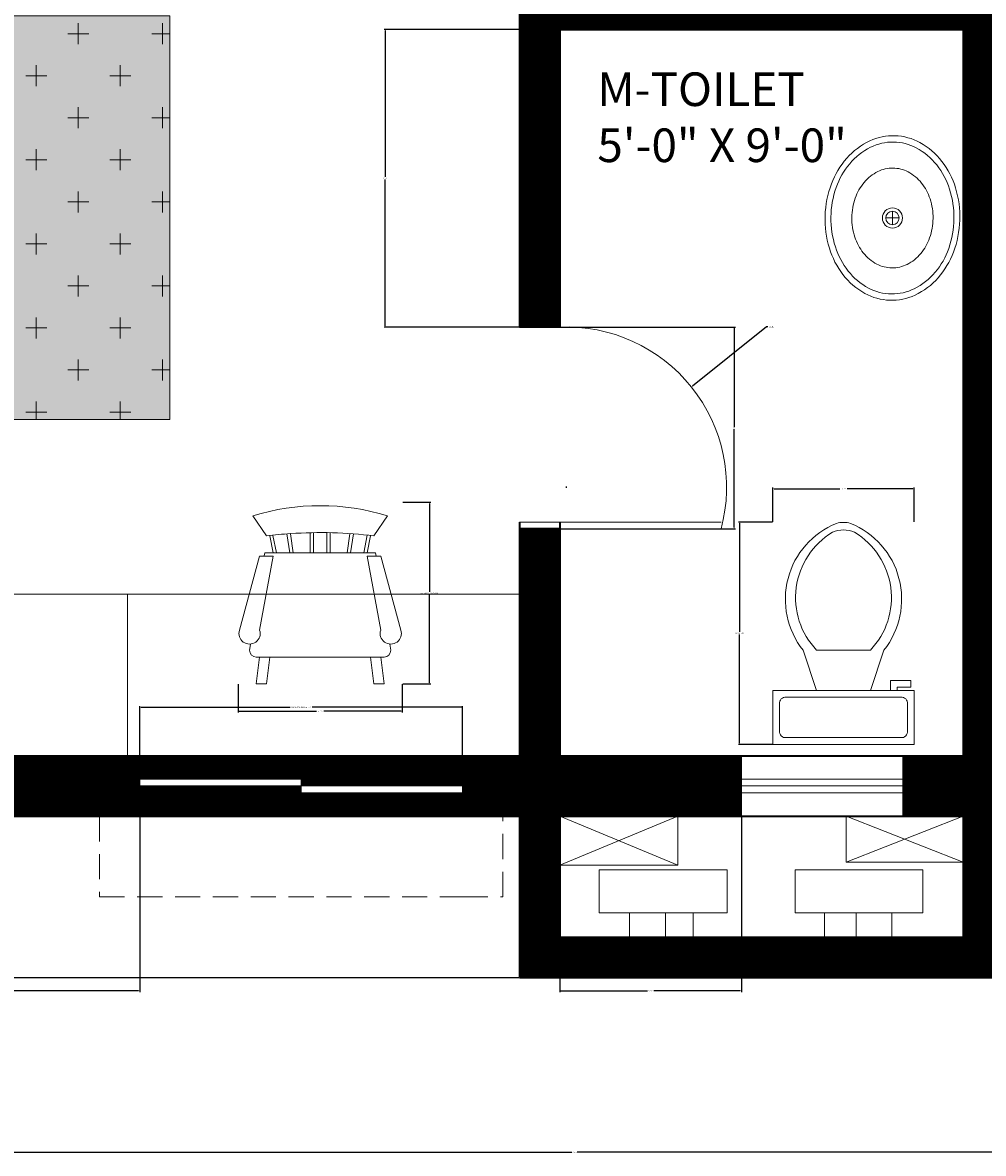
# Model space of a CAD drawing. Units: inches. Extents: x 557 to 1007, y 390 to 953.
# Tile 2 of 10: x 700 to 842, y 390 to 558. Entities that reach past the tile are written whole.
import ezdxf

# ---------------------------------------------------------------- set-up
doc = ezdxf.new("R2010")
doc.units = ezdxf.units.IN
doc.header["$LTSCALE"] = 5
doc.header["$MEASUREMENT"] = 0
doc.linetypes.add('HIDDEN', pattern=[0.375, 0.25, -0.125])
for name, color, linetype, lineweight in [('A-ANNO-DIMS', 2, 'Continuous', 18), ('A-AREA-IDEN', 7, 'Continuous', 18), ('A-DOOR', 3, 'Continuous', 18), ('A-EQPM', 8, 'Continuous', 18), ('A-FLOR-CASE', 8, 'Continuous', 18), ('A-FLOR-FIXT', 9, 'Continuous', 18), ('A-FURN', 8, 'Continuous', 18), ('A-FURN-PATT', 9, 'Continuous', 9), ('A-GLAZ', 4, 'Continuous', 18), ('A-GLAZ-OVHD', 8, 'HIDDEN', 13), ('A-WALL', 7, 'Continuous', 35)]:
    doc.layers.add(name, color=color, linetype=linetype, lineweight=lineweight)
doc.layers.add('A-GLAZ-PATT', color=141, linetype='Continuous', lineweight=9, true_color=0xadddf7)
doc.layers.add('A-WALL-PATT', color=251, linetype='Continuous', lineweight=9, true_color=0x636466)
doc.styles.get("Standard").update_dxf_attribs({"font": 'arial.ttf'})
doc.dimstyles.get("Standard").update_dxf_attribs({"dimtxt": 0.18, "dimasz": 0.18, "dimexe": 0.18, "dimexo": 0.0625, "dimgap": 0.09, "dimtad": 0, "dimtih": 1, "dimtoh": 1, "dimdec": 4, "dimzin": 0, "dimdsep": 46, "dimtxsty": 'Standard', "dimcen": 0.09, "dimadec": 0, "dimazin": 0, "dimtfac": 1, "dimtdec": 4, "dimtofl": 0, "dimtmove": 0, "dimatfit": 3, "dimfxl": 1, "dimtolj": 1, "dimtzin": 0, "dimarcsym": 0})

# ---------------------------------------------------------------- blocks, each defined once
blk = doc.blocks.new('Chair - Rocking')
for p, q in [((-8, -4.5), (-10, -1.5)), ((8, -4.5), (10, -1.5)), ((-7.5, -4.5), (-7, -7)), ((-6.5, -7), (-7.02225, -4.43)), ((-4.5, -7), (-4.96674, -4.19951)), ((-4, -7), (-4.40532, -4.16272)), ((-1.5, -4.05012), (-1.5, -7)), ((-1, -7), (-1, -4.05012)), ((1, -7), (1, -4.04655)), ((1.5, -4.05012), (1.5, -7)), ((4, -7), (4.40187, -4.18694)), ((4.5, -7), (4.96761, -4.19437)), ((6.5, -7), (7, -4.4057)), ((7.5, -4.5), (7, -7)), ((-9, -7.5), (-12, -18.49999)), ((-7, -7.5), (-9, -7.5)), ((-9, -18.49999), (-7, -7.5)), ((-8.23428, -6.99939), (-8.3093, -7.47958)), ((-8.23041, -7), (8.23915, -7)), ((7, -7.5), (9, -7.5)), ((9, -18.49999), (7, -7.5)), ((8.31071, -7.48854), (8.23449, -7.00073)), ((9, -7.5), (12, -18.49999)), ((-10.36644, -20.64523), (-10.5, -21.49999)), ((10.5, -21.49999), (10.3575, -20.58798)), ((-9, -22.49999), (-9.5, -26.49999)), ((0, -22.49999), (-9.5, -22.49999)), ((-8, -26.49999), (-7.5, -22.49999)), ((0, -22.49999), (9.5, -22.49999)), ((8, -26.49999), (7.5, -22.49999)), ((9, -22.49999), (9.5, -26.49999)), ((-9.5, -26.49999), (-8, -26.49999)), ((9.5, -26.49999), (8, -26.49999))]:
    blk.add_line(p, q)
for centre, radius, start, end in [((0, -34.08333), 34.08333, 72.93847, 107.0615), ((0, -68.25004), 64.25, 93.92211, 97.15267), ((0, -68.25004), 64.25, 82.84733, 93.92211), ((-10.5, -18.99999), 1.58114, 161.5651, 18.43495), ((10.5, -18.99999), 1.58114, 161.5651, 18.43495), ((-9.5, -21.49999), 1, 180, 270), ((9.5, -21.49999), 1, 270, 0)]:
    blk.add_arc(centre, radius, start, end)
blk = doc.blocks.new('Toilet - top')
for p, q in [((9.5, -6), (9.5, -2)), ((-8, -8.5), (-8, -8)), ((-7, -8), (-7, -9.5)), ((-4, -8), (-6, -14)), ((4, -8), (6, -14)), ((-10, -8.5), (-8, -8.5)), ((-10, -9.5), (-10, -8.5)), ((-7, -9.5), (-10, -9.5)), ((4, -14), (-4, -14))]:
    blk.add_line(p, q)
blk.add_lwpolyline([(10.5, -8), (10.5, 0), (-10.5, 0), (-10.5, -8)], close=True)
for points in [[(8.5, -1), (-8.5, -1)], [(-9.5, -2), (-9.5, -6)], [(-8.5, -7), (8.5, -7)]]:
    blk.add_lwpolyline(points)
for centre, radius, start, end in [((-8.62, -1.88), 0.884, 81.8699, 188.1301), ((8.62, -1.88), 0.884, 351.8699, 98.1301), ((-8.62, -6.12), 0.884, 171.8699, 278.1301), ((8.62, -6.12), 0.884, 261.8699, 8.1301), ((3.52, -21.58), 12.17, 141.4691, 247.9714), ((4.2, -21.82), 11.33, 136.3677, 238.9468), ((-3.52, -21.58), 12.17, 292.0284, 38.5307), ((-4.2, -21.82), 11.33, 301.053, 43.6321), ((0, -27.88), 4, 245.7318, 294.2682), ((0, -29), 4, 254.8605, 285.1395)]:
    blk.add_arc(centre, radius, start, end)
blk = doc.blocks.new('Sink - Oval top')
for p, q in [((-1, 0), (1, 0)), ((0, 1), (0, -1))]:
    blk.add_line(p, q)
for points in [[(-12.23, 0.39, 0.117634), (-11.46, -3.36, 0.104469), (-8.88, -6.8, 0.090016), (-5.08, -9.07, 0.08192), (-0.32, -10.02, 0.08192), (4.49, -9.38, 0.090016), (8.42, -7.36, 0.104469), (11.22, -4.09, 0.117634), (12.23, -0.39, 0.117634), (11.46, 3.36, 0.104469), (8.88, 6.8, 0.090016), (5.08, 9.07, 0.08192), (0.32, 10.02, 0.08192), (-4.49, 9.38, 0.090016), (-8.42, 7.36, 0.104469), (-11.22, 4.09, 0.117634)], [(-11.29, 0.16, 0.118622), (-10.52, -3.25, 0.104678), (-8.07, -6.36, 0.089562), (-4.54, -8.37, 0.081185), (-0.13, -9.15, 0.081185), (4.3, -8.49, 0.089562), (7.89, -6.58, 0.104678), (10.42, -3.55, 0.118622), (11.29, -0.16, 0.118622), (10.52, 3.25, 0.104678), (8.07, 6.36, 0.089562), (4.54, 8.37, 0.081185), (0.13, 9.15, 0.081185), (-4.3, 8.49, 0.089562), (-7.89, 6.58, 0.104678), (-10.42, 3.55, 0.118622)], [(-7.42, 0.08, 0.118283), (-6.91, -2.17, 0.104607), (-5.29, -4.21, 0.089718), (-2.97, -5.53, 0.081436), (-0.07, -6.04, 0.081436), (2.84, -5.59, 0.089718), (5.2, -4.33, 0.104607), (6.86, -2.32, 0.118283), (7.42, -0.08, 0.118283), (6.91, 2.17, 0.104607), (5.29, 4.21, 0.089718), (2.97, 5.53, 0.081436), (0.07, 6.04, 0.081436), (-2.84, 5.59, 0.089718), (-5.2, 4.33, 0.104607), (-6.86, 2.32, 0.118283)]]:
    blk.add_lwpolyline(points, format="xyb", close=True)
for radius in [1.5, 1]:
    blk.add_circle((0, 0), radius)
blk = doc.blocks.new('BED-QUEEN-60x80-PLAN')
for p, q in [((0, 0), (0, 60)), ((0, 60), (80, 60)), ((29.6, 60), (14.4, 44.8)), ((29.6, 44.8), (29.6, 60)), ((80, 60), (80, 0)), ((1.2, 52), (16.4, 52)), ((1.2, 31.2), (1.2, 52)), ((16.4, 52), (16.4, 46.8)), ((14.4, 0), (14.4, 44.8)), ((14.4, 44.8), (29.6, 44.8)), ((16.8, 44.8), (16.8, 0)), ((14.4, 31.2), (1.2, 31.2)), ((1.2, 28.8), (14.4, 28.8)), ((1.2, 8), (1.2, 28.8)), ((14.4, 8), (1.2, 8)), ((80, 0), (0, 0))]:
    blk.add_line(p, q)
blk = doc.blocks.new('WIN-24-VENT')
for p, q in [((0, 0), (0, 9)), ((24, 0), (24, 9)), ((24, 5.5), (0, 5.5)), ((24, 4.5), (0, 4.5)), ((24, 3.5), (0, 3.5))]:
    blk.add_line(p, q)
blk = doc.blocks.new('WIN-48-SLIDING')
for p, q in [((0, 9), (0, 0)), ((48, 9), (48, 0)), ((24, 5.5), (0, 5.5)), ((24, 5.5), (24, 3.5)), ((48, 4.5), (0, 4.5)), ((48, 3.5), (24, 3.5))]:
    blk.add_line(p, q)
blk = doc.blocks.new('WINDOW-SHADE-60')
at = {"ltscale": 3}
for p, q in [((12, 60), (0, 60)), ((0, 60), (0, 6)), ((12, 54), (12, 60)), ((0, 6), (0, 0)), ((0, 0), (12, 0))]:
    blk.add_line(p, q, dxfattribs=at)
blk = doc.blocks.new('*D23')
at = {"layer": 'A-ANNO-DIMS', "color": 0, "lineweight": -2, "ltscale": 5, "transparency": 16777216}
for p, q in [((756.06, 486.58), (760.23, 486.58)), ((760.05, 486.4), (760.05, 473.26)), ((760.05, 459.76), (760.05, 472.9)), ((756.06, 459.58), (760.23, 459.58))]:
    blk.add_line(p, q, dxfattribs=at)
at = {"layer": 'A-ANNO-DIMS', "color": 0, "ltscale": 5, "transparency": 16777216}
for points in [[(760.02, 486.4), (760.08, 486.4), (760.05, 486.58)], [(760.02, 459.76), (760.08, 459.76), (760.05, 459.58)]]:
    blk.add_solid(points, dxfattribs=at)
at = {"layer": 'Defpoints', "color": 0, "ltscale": 5, "transparency": 16777216}
for p in [(756, 486.58), (760.05, 486.58), (756, 459.58)]:
    blk.add_point(p, dxfattribs=at)
at = {"layer": 'A-ANNO-DIMS', "color": 0, "ltscale": 5, "transparency": 16777216, "insert": (760.05, 473.08), "char_height": 0.18, "attachment_point": 5}
blk.add_mtext('\\A1;ROCKING CHAIR 27 TYP.', dxfattribs=at)
blk = doc.blocks.new('*D24')
at = {"layer": 'A-ANNO-DIMS', "color": 0, "lineweight": -2, "ltscale": 5, "transparency": 16777216}
for p, q in [((731.57, 459.52), (731.57, 455.35)), ((756, 459.52), (756, 455.35)), ((731.75, 455.53), (743.26, 455.53)), ((755.82, 455.53), (744.31, 455.53))]:
    blk.add_line(p, q, dxfattribs=at)
at = {"layer": 'A-ANNO-DIMS', "color": 0, "ltscale": 5, "transparency": 16777216}
for points in [[(731.75, 455.56), (731.75, 455.5), (731.57, 455.53)], [(755.82, 455.56), (755.82, 455.5), (756, 455.53)]]:
    blk.add_solid(points, dxfattribs=at)
at = {"layer": 'Defpoints', "color": 0, "ltscale": 5, "transparency": 16777216}
for p in [(731.57, 459.58), (756, 459.58), (756, 455.53)]:
    blk.add_point(p, dxfattribs=at)
at = {"layer": 'A-ANNO-DIMS', "color": 0, "ltscale": 5, "transparency": 16777216, "insert": (743.78, 455.53), "char_height": 0.18, "attachment_point": 5}
blk.add_mtext('\\A1;24 TYP.', dxfattribs=at)
blk = doc.blocks.new('*D29')
at = {"layer": 'A-ANNO-DIMS', "color": 0, "lineweight": -2, "ltscale": 5, "transparency": 16777216}
for p, q in [((811.04, 483.64), (805.97, 483.64)), ((806.15, 483.46), (806.15, 467.3)), ((806.15, 450.77), (806.15, 466.93)), ((811.04, 450.59), (805.97, 450.59))]:
    blk.add_line(p, q, dxfattribs=at)
at = {"layer": 'A-ANNO-DIMS', "color": 0, "ltscale": 5, "transparency": 16777216}
for points in [[(806.12, 483.46), (806.18, 483.46), (806.15, 483.64)], [(806.12, 450.77), (806.18, 450.77), (806.15, 450.59)]]:
    blk.add_solid(points, dxfattribs=at)
at = {"layer": 'Defpoints', "color": 0, "ltscale": 5, "transparency": 16777216}
for p in [(811.1, 483.64), (806.15, 450.59), (811.1, 450.59)]:
    blk.add_point(p, dxfattribs=at)
at = {"layer": 'A-ANNO-DIMS', "color": 0, "ltscale": 5, "transparency": 16777216, "insert": (806.15, 467.11), "char_height": 0.18, "attachment_point": 5}
blk.add_mtext('\\A1;WC 33 TYP.', dxfattribs=at)
blk = doc.blocks.new('*D30')
at = {"layer": 'A-ANNO-DIMS', "color": 0, "lineweight": -2, "ltscale": 5, "transparency": 16777216}
for p, q in [((811.1, 483.7), (811.1, 488.77)), ((811.28, 488.59), (821.07, 488.59)), ((831.92, 488.59), (822.13, 488.59)), ((832.1, 483.7), (832.1, 488.77))]:
    blk.add_line(p, q, dxfattribs=at)
at = {"layer": 'A-ANNO-DIMS', "color": 0, "ltscale": 5, "transparency": 16777216}
for points in [[(811.28, 488.62), (811.28, 488.56), (811.1, 488.59)], [(831.92, 488.62), (831.92, 488.56), (832.1, 488.59)]]:
    blk.add_solid(points, dxfattribs=at)
at = {"layer": 'Defpoints', "color": 0, "ltscale": 5, "transparency": 16777216}
for p in [(811.1, 488.59), (811.1, 483.64), (832.1, 483.64)]:
    blk.add_point(p, dxfattribs=at)
at = {"layer": 'A-ANNO-DIMS', "color": 0, "ltscale": 5, "transparency": 16777216, "insert": (821.6, 488.59), "char_height": 0.18, "attachment_point": 5}
blk.add_mtext('\\A1;21 TYP.', dxfattribs=at)
blk = doc.blocks.new('*D33')
at = {"layer": 'A-ANNO-DIMS', "color": 0, "lineweight": -2, "ltscale": 5, "transparency": 16777216}
for p, q in [((716.96, 448.97), (716.96, 456.28)), ((717.14, 456.1), (739.31, 456.1)), ((764.78, 456.1), (742.61, 456.1)), ((764.96, 448.97), (764.96, 456.28))]:
    blk.add_line(p, q, dxfattribs=at)
at = {"layer": 'A-ANNO-DIMS', "color": 0, "ltscale": 5, "transparency": 16777216}
for points in [[(717.14, 456.13), (717.14, 456.07), (716.96, 456.1)], [(764.78, 456.13), (764.78, 456.07), (764.96, 456.1)]]:
    blk.add_solid(points, dxfattribs=at)
at = {"layer": 'Defpoints', "color": 0, "ltscale": 5, "transparency": 16777216}
for p in [(764.96, 456.1), (716.96, 448.9), (764.96, 448.9)]:
    blk.add_point(p, dxfattribs=at)
at = {"layer": 'A-ANNO-DIMS', "color": 0, "ltscale": 5, "transparency": 16777216, "insert": (740.96, 456.1), "char_height": 0.18, "attachment_point": 5}
blk.add_mtext('\\A1;SLIDING WINDOW 48 TYP.', dxfattribs=at)
blk = doc.blocks.new('*D34')
at = {"layer": 'A-ANNO-DIMS', "color": 0, "lineweight": -2, "ltscale": 5, "transparency": 16777216}
for p, q in [((716.9, 448.9), (709.58, 448.9)), ((709.76, 448.72), (709.76, 444.59)), ((709.76, 440.08), (709.76, 444.22)), ((716.9, 439.9), (709.58, 439.9))]:
    blk.add_line(p, q, dxfattribs=at)
at = {"layer": 'A-ANNO-DIMS', "color": 0, "ltscale": 5, "transparency": 16777216}
for points in [[(709.73, 448.72), (709.79, 448.72), (709.76, 448.9)], [(709.73, 440.08), (709.79, 440.08), (709.76, 439.9)]]:
    blk.add_solid(points, dxfattribs=at)
at = {"layer": 'Defpoints', "color": 0, "ltscale": 5, "transparency": 16777216}
for p in [(709.76, 448.9), (716.96, 448.9), (716.96, 439.9)]:
    blk.add_point(p, dxfattribs=at)
at = {"layer": 'A-ANNO-DIMS', "color": 0, "ltscale": 5, "transparency": 16777216, "insert": (709.76, 444.4), "char_height": 0.18, "attachment_point": 5}
blk.add_mtext('\\A1;9 TYP.', dxfattribs=at)
blk = doc.blocks.new('*D45')
at = {"layer": 'A-ANNO-DIMS', "color": 0, "lineweight": -2, "ltscale": 5, "transparency": 16777216}
for p, q in [((582.82, 605.84), (582.82, 389.77)), ((980.41, 439.84), (980.41, 389.77)), ((583, 389.95), (781.22, 389.95)), ((980.23, 389.95), (782.01, 389.95))]:
    blk.add_line(p, q, dxfattribs=at)
at = {"layer": 'A-ANNO-DIMS', "color": 0, "ltscale": 5, "transparency": 16777216}
for points in [[(583, 389.98), (583, 389.92), (582.82, 389.95)], [(980.23, 389.98), (980.23, 389.92), (980.41, 389.95)]]:
    blk.add_solid(points, dxfattribs=at)
at = {"layer": 'Defpoints', "color": 0, "ltscale": 5, "transparency": 16777216}
for p in [(582.82, 605.9), (980.41, 439.9), (980.41, 389.95)]:
    blk.add_point(p, dxfattribs=at)
at = {"layer": 'A-ANNO-DIMS', "color": 0, "ltscale": 5, "transparency": 16777216, "insert": (781.61, 389.95), "char_height": 0.18, "attachment_point": 5}
blk.add_mtext('\\A1;397.6', dxfattribs=at)
blk = doc.blocks.new('*D46')
at = {"layer": 'A-ANNO-DIMS', "color": 0, "lineweight": -2, "ltscale": 5, "transparency": 16777216}
for p, q in [((761.34, 926.9), (556.69, 926.9)), ((556.87, 926.72), (556.87, 671.59)), ((556.87, 416.08), (556.87, 671.22)), ((773.34, 415.9), (556.69, 415.9))]:
    blk.add_line(p, q, dxfattribs=at)
at = {"layer": 'A-ANNO-DIMS', "color": 0, "ltscale": 5, "transparency": 16777216}
for points in [[(556.84, 926.72), (556.9, 926.72), (556.87, 926.9)], [(556.84, 416.08), (556.9, 416.08), (556.87, 415.9)]]:
    blk.add_solid(points, dxfattribs=at)
at = {"layer": 'Defpoints', "color": 0, "ltscale": 5, "transparency": 16777216}
for p in [(556.87, 926.9), (761.41, 926.9), (773.41, 415.9)]:
    blk.add_point(p, dxfattribs=at)
at = {"layer": 'A-ANNO-DIMS', "color": 0, "ltscale": 5, "transparency": 16777216, "insert": (556.87, 671.4), "char_height": 0.18, "attachment_point": 5}
blk.add_mtext('\\A1;511', dxfattribs=at)
blk = doc.blocks.new('*D68')
at = {"layer": 'A-ANNO-DIMS', "color": 0, "lineweight": -2, "ltscale": 5, "transparency": 16777216}
for p, q in [((632.41, 439.84), (632.41, 413.77)), ((716.96, 439.84), (716.96, 413.77)), ((632.59, 413.95), (674.29, 413.95)), ((716.78, 413.95), (675.08, 413.95))]:
    blk.add_line(p, q, dxfattribs=at)
at = {"layer": 'A-ANNO-DIMS', "color": 0, "ltscale": 5, "transparency": 16777216}
for points in [[(632.59, 413.98), (632.59, 413.92), (632.41, 413.95)], [(716.78, 413.98), (716.78, 413.92), (716.96, 413.95)]]:
    blk.add_solid(points, dxfattribs=at)
at = {"layer": 'Defpoints', "color": 0, "ltscale": 5, "transparency": 16777216}
for p in [(632.41, 439.9), (716.96, 439.9), (632.41, 413.95)]:
    blk.add_point(p, dxfattribs=at)
at = {"layer": 'A-ANNO-DIMS', "color": 0, "ltscale": 5, "transparency": 16777216, "insert": (674.68, 413.95), "char_height": 0.18, "attachment_point": 5}
blk.add_mtext('\\A1;84.55', dxfattribs=at)
blk = doc.blocks.new('*D73')
at = {"layer": 'A-ANNO-DIMS', "color": 0, "lineweight": -2, "ltscale": 5, "transparency": 16777216}
for p, q in [((779.47, 512.64), (805.54, 512.64)), ((805.36, 512.46), (805.36, 497.82)), ((805.36, 482.82), (805.36, 497.45)), ((779.47, 482.64), (805.54, 482.64))]:
    blk.add_line(p, q, dxfattribs=at)
at = {"layer": 'A-ANNO-DIMS', "color": 0, "ltscale": 5, "transparency": 16777216}
for points in [[(805.33, 512.46), (805.39, 512.46), (805.36, 512.64)], [(805.33, 482.82), (805.39, 482.82), (805.36, 482.64)]]:
    blk.add_solid(points, dxfattribs=at)
at = {"layer": 'Defpoints', "color": 0, "ltscale": 5, "transparency": 16777216}
for p in [(779.41, 512.64), (779.41, 482.64), (805.36, 482.64)]:
    blk.add_point(p, dxfattribs=at)
at = {"layer": 'A-ANNO-DIMS', "color": 0, "ltscale": 5, "transparency": 16777216, "insert": (805.36, 497.64), "char_height": 0.18, "attachment_point": 5}
blk.add_mtext('\\A1;30', dxfattribs=at)
blk = doc.blocks.new('*D77')
at = {"layer": 'A-ANNO-DIMS', "color": 0, "lineweight": -2, "ltscale": 5, "transparency": 16777216}
for p, q in [((779.41, 439.84), (779.41, 413.77)), ((806.43, 439.84), (806.43, 413.77)), ((779.59, 413.95), (792.45, 413.95)), ((806.25, 413.95), (793.38, 413.95))]:
    blk.add_line(p, q, dxfattribs=at)
at = {"layer": 'A-ANNO-DIMS', "color": 0, "ltscale": 5, "transparency": 16777216}
for points in [[(779.59, 413.98), (779.59, 413.92), (779.41, 413.95)], [(806.25, 413.98), (806.25, 413.92), (806.43, 413.95)]]:
    blk.add_solid(points, dxfattribs=at)
at = {"layer": 'Defpoints', "color": 0, "ltscale": 5, "transparency": 16777216}
for p in [(779.41, 439.9), (806.43, 439.9), (779.41, 413.95)]:
    blk.add_point(p, dxfattribs=at)
at = {"layer": 'A-ANNO-DIMS', "color": 0, "ltscale": 5, "transparency": 16777216, "insert": (792.92, 413.95), "char_height": 0.18, "attachment_point": 5}
blk.add_mtext('\\A1;27.027', dxfattribs=at)
blk = doc.blocks.new('*D93')
at = {"layer": 'A-ANNO-DIMS', "color": 0, "lineweight": -2, "ltscale": 5, "transparency": 16777216}
for p, q in [((773.41, 512.7), (773.41, 538.77)), ((773.59, 538.59), (776.26, 538.59)), ((779.23, 538.59), (776.55, 538.59)), ((779.41, 512.7), (779.41, 538.77))]:
    blk.add_line(p, q, dxfattribs=at)
at = {"layer": 'A-ANNO-DIMS', "color": 0, "ltscale": 5, "transparency": 16777216}
for points in [[(773.59, 538.62), (773.59, 538.56), (773.41, 538.59)], [(779.23, 538.62), (779.23, 538.56), (779.41, 538.59)]]:
    blk.add_solid(points, dxfattribs=at)
at = {"layer": 'Defpoints', "color": 0, "ltscale": 5, "transparency": 16777216}
for p in [(779.41, 538.59), (773.41, 512.64), (779.41, 512.64)]:
    blk.add_point(p, dxfattribs=at)
at = {"layer": 'A-ANNO-DIMS', "color": 0, "ltscale": 5, "transparency": 16777216, "insert": (776.41, 538.59), "char_height": 0.18, "attachment_point": 5}
blk.add_mtext('\\A1;6', dxfattribs=at)
blk = doc.blocks.new('*D94')
at = {"layer": 'A-ANNO-DIMS', "color": 0, "lineweight": -2, "ltscale": 5, "transparency": 16777216}
for p, q in [((779.34, 556.9), (753.28, 556.9)), ((753.46, 556.72), (753.46, 534.95)), ((753.46, 512.82), (753.46, 534.59)), ((779.34, 512.64), (753.28, 512.64))]:
    blk.add_line(p, q, dxfattribs=at)
at = {"layer": 'A-ANNO-DIMS', "color": 0, "ltscale": 5, "transparency": 16777216}
for points in [[(753.43, 556.72), (753.49, 556.72), (753.46, 556.9)], [(753.43, 512.82), (753.49, 512.82), (753.46, 512.64)]]:
    blk.add_solid(points, dxfattribs=at)
at = {"layer": 'Defpoints', "color": 0, "ltscale": 5, "transparency": 16777216}
for p in [(753.46, 556.9), (779.41, 556.9), (779.41, 512.64)]:
    blk.add_point(p, dxfattribs=at)
at = {"layer": 'A-ANNO-DIMS', "color": 0, "ltscale": 5, "transparency": 16777216, "insert": (753.46, 534.77), "char_height": 0.18, "attachment_point": 5}
blk.add_mtext('\\A1;44.27', dxfattribs=at)
blk = doc.blocks.new('*D111')
at = {"layer": 'A-ANNO-DIMS', "color": 0, "lineweight": -2, "ltscale": 5, "transparency": 16777216}
for p, q in [((810.17, 512.65), (799.14, 503.83)), ((810.35, 512.65), (810.17, 512.65)), ((780.3, 488.83), (780.48, 488.83)), ((780.39, 488.74), (780.39, 488.92))]:
    blk.add_line(p, q, dxfattribs=at)
at = {"layer": 'A-ANNO-DIMS', "color": 0, "ltscale": 5, "transparency": 16777216}
blk.add_solid([(799.12, 503.85), (799.16, 503.8), (799, 503.71)], dxfattribs=at)
at = {"layer": 'Defpoints', "color": 0, "ltscale": 5, "transparency": 16777216}
for p in [(799, 503.71), (780.39, 488.83)]:
    blk.add_point(p, dxfattribs=at)
at = {"layer": 'A-ANNO-DIMS', "color": 0, "ltscale": 5, "transparency": 16777216, "insert": (810.83, 512.65), "char_height": 0.18, "attachment_point": 5}
blk.add_mtext('\\A1;R23.83', dxfattribs=at)

msp = doc.modelspace()

# ---------------------------------------------------------------- hatches: boundary and pattern name
at = {"layer": 'A-FURN-PATT', "ltscale": 5}
h = msp.add_hatch(dxfattribs=at)
h.set_pattern_fill('GRAVEL', color=256, scale=25)
h.set_pattern_definition([(228.01279, (18, 25), (-200, -225), [3.3634, -332.9772]), (184.96974, (15.75, 22.5), (300, 25), [5.7717, -571.39812]), (132.51045, (10, 22), (250, -275), [4.0697, -402.9008]), (267.27369, (0.25, 15.75), (25, 500), [5.25595, -520.33895]), (292.83365, (0, 10.5), (-125, 300), [5.15387, -510.23433]), (357.27369, (2, 5.75), (-500, 25), [5.25595, -520.33895]), (37.69424, (7.25, 5.5), (-325, -250), [6.95072, -688.1212]), (72.25533, (12.75, 9.75), (175, 550), [6.5622, -649.65804]), (121.42957, (14.75, 16), (-200, 325), [5.27375, -522.10183]), (175.23636, (12, 20.5), (275, -25), [6.0208, -295.01906]), (222.39744, (6, 21), (-300, -275), [7.7862, -770.83438]), (138.81407, (25, 15.5), (-175, 150), [2.65752, -263.0961]), (171.46923, (23, 17.25), (325, -50), [5.05593, -500.5378]), (225, (18, 18), (-3e-15, -25), [3.53552, -31.8198]), (203.1986, (16.25, 21), (125, 50), [1.90395, -188.49038]), (291.8014, (14.5, 20.25), (-25, 75), [2.69257, -131.93655]), (30.96376, (15.5, 17.75), (75, 50), [4.37322, -141.40057]), (161.56505, (19.25, 20), (50, -25), [3.16228, -75.89467]), (16.38954, (0, 20.25), (250, 75), [4.43, -438.57113]), (70.34618, (4.25, 21.5), (-100, -275), [3.71652, -367.9352]), (293.1986, (19.25, 25), (-50, 125), [3.80788, -186.58645]), (343.61046, (20.75, 21.5), (-250, 75), [4.43, -438.57113]), (339.44395, (0, 4.75), (-125, 50), [4.272, -209.3281]), (294.77514, (4, 3.25), (-125, 275), [3.57945, -354.36608]), (66.8014, (19.5, 0), (50, 125), [3.80788, -186.58645]), (17.35402, (21, 3.5), (-325, -100), [4.19078, -414.8856]), (69.44395, (7.25, 0), (-50, -125), [2.136, -211.4641]), (101.30993, (18, 0), (-25, 100), [1.27475, -126.20074]), (165.96376, (17.75, 1.25), (75, -25), [5.15388, -97.92377]), (186.00901, (12.75, 2.5), (250, 25), [4.77625, -472.84808]), (303.69007, (15.5, 15.5), (-25, 50), [3.60555, -86.53323]), (353.15723, (17.5, 12.5), (425, -50), [6.29485, -623.18907]), (60.9454, (23.75, 11.75), (-100, -175), [2.5739, -254.81685]), (90, (25, 14), (-25, 25), [1.5, -23.5]), (120.25644, (12.25, 3.25), (100, -175), [3.4731, -343.838]), (48.01279, (10.5, 6.25), (200, 225), [6.7268, -329.6138]), (0, (15, 11.25), (25, 25), [6.5, -18.5]), (325.30485, (21.5, 11.25), (250, -175), [3.95285, -391.33186]), (254.0546, (24.75, 9), (-25, -100), [3.64005, -178.3627]), (207.64598, (23.75, 5.5), (-475, -250), [5.92662, -586.73685]), (175.42608, (18.5, 2.75), (-325, 25), [6.26997, -620.72684])])
h.paths.add_polyline_path([(615.2525, 688.5, 1), (640.7475, 688.5, 1)])
h.paths.add_polyline_path([(917.0544, 663.8414, 0.33333323), (915.2241, 665.6717), (882.2793, 665.6717, 0.33333323), (880.449, 663.8414), (880.449, 649.1992, 0.33333323), (882.2793, 647.369), (915.2241, 647.369, 0.33333323), (917.0544, 649.1992)])
h.paths.add_polyline_path([(828.0807, 699.7098), (756.0807, 699.7098), (756.0807, 663.7098), (828.0807, 663.7098)])
h.paths.add_polyline_path([(787.5651, 663.7098), (768.5964, 663.7098), (769.8463, 655.7098), (786.3151, 655.7098)])
h.paths.add_polyline_path([(815.5651, 663.7098), (796.5964, 663.7098), (797.8463, 655.7098), (814.3151, 655.7098)])
h.paths.add_polyline_path([(836.0807, 689.9442), (828.0807, 691.1942), (828.0807, 672.2255), (836.0807, 673.4755)])
h.paths.add_polyline_path([(756.0807, 691.1942), (748.0807, 689.9442), (748.0807, 673.4755), (756.0807, 672.2255)])
h.paths.add_polyline_path([(786.3151, 707.7098), (769.8463, 707.7098), (768.5964, 699.7098), (787.5651, 699.7098)])
h.paths.add_polyline_path([(814.3151, 707.7098), (797.8463, 707.7098), (796.5964, 699.7098), (815.5651, 699.7098)])
h.paths.add_polyline_path([(917.4362, 607.3575), (889.5896, 607.3575), (889.5896, 586.4726), (917.4362, 586.4726)])
h.paths.add_polyline_path([(721.4053, 881.8539), (671.0053, 881.8539), (671.0053, 866.6539), (658.2053, 866.6539), (658.2053, 821.8539), (721.4053, 821.8539)])
h.paths.add_polyline_path([(925.4053, 875.1046), (875.0053, 875.1046), (875.0053, 859.9046), (862.2053, 859.9046), (862.2053, 815.1046), (925.4053, 815.1046)])
h.paths.add_polyline_path([(721.4053, 558.9046), (671.0053, 558.9046), (671.0053, 543.7046), (658.2053, 543.7046), (658.2053, 498.9046), (721.4053, 498.9046)])
at = {"layer": 'A-FURN-PATT'}
h = msp.add_hatch(dxfattribs=at)
h.set_pattern_fill('CROSS', color=256, scale=25)
h.paths.add_polyline_path([(925.4053, 875.1046), (875.0053, 875.1046), (875.0053, 859.9046), (862.2053, 859.9046), (862.2053, 815.1046), (925.4053, 815.1046)])
h.paths.add_polyline_path([(721.4053, 881.8539), (671.0053, 881.8539), (671.0053, 866.6539), (658.2053, 866.6539), (658.2053, 821.8539), (721.4053, 821.8539)])
h.paths.add_polyline_path([(671.0053, 881.8539), (655.8053, 866.6539), (671.0053, 866.6539)], flags=17)
h.paths.add_polyline_path([(671.0053, 881.8539), (641.4053, 881.8539), (641.4053, 821.8539), (655.8053, 821.8539), (655.8053, 829.8539), (642.6053, 829.8539), (642.6053, 850.6539), (655.8053, 850.6539), (655.8053, 853.0539), (642.6053, 853.0539), (642.6053, 873.8539), (657.8053, 873.8539), (657.8053, 868.6539)])
h.paths.add_polyline_path([(875.0053, 875.1046), (859.8053, 859.9046), (875.0053, 859.9046)], flags=17)
h.paths.add_polyline_path([(875.0053, 875.1046), (845.4053, 875.1046), (845.4053, 815.1046), (859.8053, 815.1046), (859.8053, 823.1046), (846.6053, 823.1046), (846.6053, 843.9046), (859.8053, 843.9046), (859.8053, 846.3046), (846.6053, 846.3046), (846.6053, 867.1046), (861.8053, 867.1046), (861.8053, 861.9046)])
h.paths.add_polyline_path([(721.4053, 558.9046), (671.0053, 558.9046), (671.0053, 543.7046), (658.2053, 543.7046), (658.2053, 498.9046), (721.4053, 498.9046)])
h.paths.add_polyline_path([(671.0053, 558.9046), (641.4053, 558.9046), (641.4053, 498.9046), (655.8053, 498.9046), (655.8053, 506.9046), (642.6053, 506.9046), (642.6053, 527.7046), (655.8053, 527.7046), (655.8053, 530.1046), (642.6053, 530.1046), (642.6053, 550.9046), (657.8053, 550.9046), (657.8053, 545.7046)])
h.paths.add_polyline_path([(671.0053, 558.9046), (657.8053, 545.7046), (655.8053, 543.7046), (671.0053, 543.7046)], flags=17)
h.paths.add_polyline_path([(873.1461, 661.8773, 0.41421356), (868.1461, 666.8773, -0.12244426), (867.1516, 666.8773), (855.014, 666.8773), (855.014, 647.2429), (867.4581, 647.2429, -0.08537395), (868.1461, 647.2429, 0.41421356), (873.1461, 652.2429)])
h.paths.add_polyline_path([(917.0544, 663.8414, 0.33333323), (915.2241, 665.6717), (882.2793, 665.6717, 0.33333323), (880.449, 663.8414), (880.449, 649.1992, 0.33333323), (882.2793, 647.369), (915.2241, 647.369, 0.33333323), (917.0544, 649.1992)])
h.paths.add_polyline_path([(944.9465, 667.5202), (932.6561, 667.5202, -0.10407786), (931.8144, 667.5202, 0.41421356), (926.8144, 662.5202), (926.8144, 652.8858, 0.41421356), (931.8144, 647.8858, -0.05611627), (932.2647, 647.8858), (944.9465, 647.8858)])
h.paths.add_polyline_path([(928.8341, 635.542, 0.41421356), (923.8341, 640.542), (914.1997, 640.542, 0.41421356), (909.1997, 635.542), (909.1997, 622.4099), (923.8341, 622.4099, 0.41421356), (928.8341, 627.4099)])
h.paths.add_polyline_path([(909.1997, 635.542, 0.41421356), (904.1997, 640.542), (894.5653, 640.542, 0.41421356), (889.5653, 635.542), (889.5653, 622.4099), (909.1997, 622.4099)])
h.paths.add_polyline_path([(889.5653, 635.542, 0.41421356), (884.5653, 640.542), (874.9308, 640.542, 0.41421356), (869.9308, 635.542), (869.9308, 627.4099, 0.41421356), (874.9308, 622.4099), (889.5653, 622.4099)])
at = {"layer": 'A-GLAZ-PATT'}
h = msp.add_hatch(dxfattribs=at)
h.set_pattern_fill('ANSI31', color=256)
h.paths.add_polyline_path([(635.9053, 814.7688), (636.9053, 814.7688), (636.9053, 838.7688), (632.4053, 838.7688), (632.4053, 790.7688), (635.9053, 790.7688)])
h.paths.add_polyline_path([(641.4053, 838.7688), (637.9053, 838.7688), (637.9053, 814.7688), (636.9053, 814.7688), (636.9053, 790.7688), (641.4053, 790.7688)])
h.paths.add_polyline_path([(603.4053, 728.9046, -0.41421356), (623.4053, 748.9046), (632.4053, 748.9046), (632.4053, 752.9046), (623.4053, 752.9046, 0.41421356), (599.4053, 728.9046), (599.4053, 614.9046), (603.4053, 614.9046)])
h.paths.add_polyline_path([(632.4053, 743.9046), (632.4053, 747.9046), (623.4053, 747.9046, 0.41421356), (604.4053, 728.9046), (604.4053, 614.9046), (608.4053, 614.9046), (608.4053, 719.9046, -0.41421356)])
h.paths.add_polyline_path([(683.4053, 722.9046), (678.9053, 722.9046), (678.9053, 698.9046), (679.9053, 698.9046), (679.9053, 662.9046), (678.9053, 662.9046), (678.9053, 638.9046), (683.4053, 638.9046)])
h.paths.add_polyline_path([(678.9053, 698.9046), (677.9053, 698.9046), (677.9053, 722.9046), (674.4053, 722.9046), (674.4053, 638.9046), (677.9053, 638.9046), (677.9053, 662.9046), (678.9053, 662.9046)])
h.paths.add_polyline_path([(635.9053, 593.9046), (632.4053, 593.9046), (632.4053, 557.9046), (635.9053, 557.9046)])
h.paths.add_polyline_path([(641.4053, 593.9046), (637.9053, 593.9046), (637.9053, 557.9046), (641.4053, 557.9046)])
h.paths.add_polyline_path([(764.9579, 448.9046), (716.9579, 448.9046), (716.9579, 445.4046), (740.9579, 445.4046), (740.9579, 444.4046), (764.9579, 444.4046)])
h.paths.add_polyline_path([(764.9579, 443.4046), (740.9579, 443.4046), (740.9579, 444.4046), (716.9579, 444.4046), (716.9579, 439.9046), (764.9579, 439.9046)])
h.paths.add_polyline_path([(938.4053, 905.9046), (878.4053, 905.9046), (878.4053, 902.4046), (908.4053, 902.4046), (908.4053, 901.4046), (938.4053, 901.4046)])
h.paths.add_polyline_path([(938.4053, 900.4046), (908.4053, 900.4046), (908.4053, 901.4046), (878.4053, 901.4046), (878.4053, 896.9046), (938.4053, 896.9046)])
h.paths.add_polyline_path([(724.9087, 905.9046), (676.9087, 905.9046), (676.9087, 902.4046), (701.4053, 902.4046), (701.4053, 901.4046), (724.9087, 901.4046)])
h.paths.add_polyline_path([(724.9087, 900.4046), (701.4053, 900.4046), (701.4053, 901.4046), (676.9087, 901.4046), (676.9087, 896.9046), (724.9087, 896.9046)])
h.paths.add_polyline_path([(832.0625, 905.9046), (808.0625, 905.9046), (808.0625, 902.4046), (832.0625, 902.4046)])
h.paths.add_polyline_path([(832.0625, 900.4046), (808.0625, 900.4046), (808.0625, 896.9046), (832.0625, 896.9046)])
at = {"layer": 'A-WALL-PATT'}
h = msp.add_hatch(dxfattribs=at)
h.set_pattern_fill('ANSI31', color=256)
h.paths.add_polyline_path([(808.0625, 905.9046), (767.4053, 905.9046), (767.4053, 920.9046), (839.4053, 920.9046), (839.4053, 905.9046), (832.0625, 905.9046), (832.0625, 896.9046), (839.4053, 896.9046), (839.4053, 800.9046), (837.4053, 800.9046), (837.4053, 794.9046), (839.4053, 794.9046), (839.4053, 790.9046), (845.4053, 790.9046), (845.4053, 896.9046), (878.4053, 896.9046), (878.4053, 905.9046), (845.4053, 905.9046), (845.4053, 926.9046), (761.4053, 926.9046), (761.4053, 914.9046), (761.4053, 905.9046), (724.9087, 905.9046), (724.9087, 896.9046), (761.4053, 896.9046), (761.4053, 752.9046), (759.4053, 752.9046), (759.4053, 746.9046), (767.4053, 746.9046), (767.4053, 794.9046), (807.4053, 794.9046), (807.4053, 800.9046), (767.4053, 800.9046), (767.4053, 896.9046), (808.0625, 896.9046)])
h.paths.add_polyline_path([(676.9087, 905.9046), (632.4053, 905.9046), (632.4053, 838.7688), (641.4053, 838.7688), (641.4053, 881.8539), (641.4053, 896.9046), (676.9087, 896.9046)])
h.paths.add_polyline_path([(980.4053, 905.9046), (938.4053, 905.9046), (938.4053, 896.9046), (971.4053, 896.9046), (971.4053, 752.9046), (845.4053, 752.9046), (845.4053, 754.9046), (839.4053, 754.9046), (839.4053, 746.9046), (971.4053, 746.9046), (971.4053, 720.1788), (980.4053, 720.1788)])
h.paths.add_polyline_path([(723.4053, 752.9046), (641.4053, 752.9046), (641.4053, 790.7688), (632.4053, 790.7688), (632.4053, 743.9046), (674.4053, 743.9046), (674.4053, 722.9046), (683.4053, 722.9046), (683.4053, 746.9046), (723.4053, 746.9046)])
h.paths.add_polyline_path([(980.4053, 684.1788), (971.4053, 684.1788), (971.4053, 614.9046), (845.4053, 614.9046), (845.4053, 608.9046), (971.4053, 608.9046), (971.4053, 512.9046), (908.7697, 512.9046), (908.7697, 508.9046), (971.4053, 508.9046), (971.4053, 448.9046), (845.4053, 448.9046), (845.4053, 508.9046), (878.7697, 508.9046), (878.7697, 512.9046), (845.4053, 512.9046), (845.4053, 562.9046), (779.4053, 562.9046), (779.4053, 614.9046), (761.4053, 614.9046), (761.4053, 608.9046), (773.4053, 608.9046), (773.4053, 512.636), (779.4053, 512.636), (779.4053, 556.9046), (839.4053, 556.9046), (839.4053, 448.9046), (830.432, 448.9046), (830.432, 439.9046), (839.4053, 439.9046), (839.4053, 433.0506), (839.4053, 421.9046), (779.4053, 421.9046), (779.4053, 439.9046), (796.9656, 439.9046), (806.432, 439.9046), (806.432, 448.9046), (779.4053, 448.9046), (779.4053, 482.636), (773.4053, 482.636), (773.4053, 448.9046), (764.9579, 448.9046), (764.9579, 439.9046), (773.4053, 439.9046), (773.4053, 415.9046), (845.4053, 415.9046), (845.4053, 439.9046), (980.4053, 439.9046)])
h.paths.add_polyline_path([(716.9579, 448.9046), (641.4053, 448.9046), (641.4053, 557.9046), (632.4053, 557.9046), (632.4053, 439.9046), (716.9579, 439.9046)])
h.paths.add_polyline_path([(725.4053, 614.9046), (683.4053, 614.9046), (683.4053, 638.9046), (674.4053, 638.9046), (674.4053, 614.9046), (608.4053, 614.9046), (582.8236, 614.9046), (582.8236, 605.9046), (599.4053, 605.9046), (632.4053, 605.9046), (641.4053, 605.9046), (641.4053, 608.9046), (725.4053, 608.9046)])
h.paths.add_polyline_path([(641.4053, 605.9046), (632.4053, 605.9046), (632.4053, 593.9046), (641.4053, 593.9046)])

# ---------------------------------------------------------------- linework, layer by layer
at = {"layer": 'A-DOOR'}
for p, q in [((773.4053, 483.636), (803.4053, 483.636)), ((773.4053, 482.636), (803.4053, 482.636))]:
    msp.add_line(p, q, dxfattribs=at)
msp.add_arc((780.3948, 488.8277), 23.8289, 344.939518, 92.380098, dxfattribs=at)
at = {"layer": 'A-EQPM'}
for p, q in [((796.9656, 432.6338), (779.4053, 439.9046)), ((796.9656, 439.9046), (779.4053, 432.6338)), ((821.9856, 439.9046), (839.4053, 433.0506)), ((839.4053, 439.9046), (821.9856, 433.0506)), ((789.7782, 421.9046), (789.7782, 425.5394)), ((795.1195, 421.9046), (795.1195, 425.5394)), ((799.2282, 421.9046), (799.2282, 425.5394)), ((818.7854, 421.9046), (818.7854, 425.5394)), ((823.4693, 421.9046), (823.4693, 425.5394)), ((828.8106, 421.9046), (828.8106, 425.5394))]:
    msp.add_line(p, q, dxfattribs=at)
for points in [[(779.4053, 439.9046), (796.9656, 439.9046), (796.9656, 432.6338), (779.4053, 432.6338)], [(839.4053, 439.9046), (821.9856, 439.9046), (821.9856, 433.0506), (839.4053, 433.0506)], [(785.2898, 425.5394), (804.2961, 425.5394), (804.2961, 431.9552), (785.2898, 431.9552)], [(814.4157, 425.5394), (833.422, 425.5394), (833.422, 431.9552), (814.4157, 431.9552)]]:
    msp.add_lwpolyline(points, close=True, dxfattribs=at)
at = {"layer": 'A-FLOR-CASE'}
for p, q in [((641.4053, 472.9046), (773.4053, 472.9046)), ((715.1542, 448.9046), (715.1542, 472.9046))]:
    msp.add_line(p, q, dxfattribs=at)
at = {"layer": 'A-WALL'}
for p, q in [((773.4053, 608.9046), (773.4053, 512.636)), ((779.4053, 556.9046), (839.4053, 556.9046)), ((779.4053, 556.9046), (779.4053, 512.636)), ((839.4053, 556.9046), (839.4053, 448.9046)), ((779.4053, 512.636), (773.4053, 512.636)), ((773.4053, 483.636), (773.4053, 448.9046)), ((779.4053, 482.636), (773.4053, 482.636)), ((779.4053, 483.636), (779.4053, 448.9046)), ((641.4053, 448.9046), (773.4053, 448.9046)), ((779.4053, 448.9046), (839.4053, 448.9046)), ((632.4053, 439.9046), (773.4053, 439.9046)), ((773.4053, 439.9046), (773.4053, 415.9046)), ((779.4053, 439.9046), (779.4053, 421.9046)), ((779.4053, 439.9046), (839.4053, 439.9046)), ((839.4053, 439.9046), (839.4053, 421.9046)), ((779.4053, 421.9046), (839.4053, 421.9046)), ((773.4053, 415.9046), (845.4053, 415.9046))]:
    msp.add_line(p, q, dxfattribs=at)

# ---------------------------------------------------------------- block references
at = {"layer": 'A-FLOR-FIXT'}
for name, p, rotation in [('Sink - Oval top', (828.8822, 528.8548), 90), ('Toilet - top', (821.604, 450.5914), 180)]:
    msp.add_blockref(name, p, dxfattribs=dict(at, rotation=rotation))
at = {"layer": 'A-FURN'}
for name, p in [('BED-QUEEN-60x80-PLAN', (641.405, 498.905)), ('Chair - Rocking', (743.7848, 486.0796))]:
    msp.add_blockref(name, p, dxfattribs=at)
at = {"layer": 'A-GLAZ'}
for name, p in [('WIN-48-SLIDING', (716.958, 439.905)), ('WIN-24-VENT', (806.4315, 439.905))]:
    msp.add_blockref(name, p, dxfattribs=at)
at = {"layer": 'A-GLAZ-OVHD', "rotation": 90.00000000000011}
msp.add_blockref('WINDOW-SHADE-60', (770.9577, 427.9043), dxfattribs=at)

# ---------------------------------------------------------------- texts
at = {"layer": 'A-AREA-IDEN', "insert": (785, 550.5), "char_height": 5, "attachment_point": 1}
msp.add_mtext_dynamic_manual_height_columns('M-TOILET\\P5\'-0" X 9\'-0"', width=125, gutter_width=1, heights=[0], dxfattribs=at)

# ---------------------------------------------------------------- dimensions: what is measured, and where the dimension line sits
at = {"layer": 'A-ANNO-DIMS', "ltscale": 5}
for base, p1, p2, angle, override, picture, middle in [((556.8736, 926.9046), (773.4053, 415.9046), (761.4053, 926.9046), 90, {"dimdec": 0, "dimlfac": 1, "dimrnd": 0, "dimzin": 0, "dimdsep": 46, "dimlunit": 2}, '*D46', (556.8736, 671.4046)), ((753.4553, 556.9046), (779.4053, 512.636), (779.4053, 556.9046), 90, {"dimdec": 2, "dimlfac": 1, "dimrnd": 0, "dimzin": 0, "dimdsep": 46, "dimlunit": 2}, '*D94', (753.4553, 534.7703)), ((805.3553, 482.636), (779.4053, 512.636), (779.4053, 482.636), 270, {"dimdec": 0, "dimlfac": 1, "dimrnd": 0, "dimzin": 0, "dimdsep": 46, "dimlunit": 2}, '*D73', (805.3553, 497.636)), ((632.4053, 413.9546), (716.9579, 439.9046), (632.4053, 439.9046), 180, {"dimdec": 2, "dimlfac": 1, "dimrnd": 0, "dimzin": 0, "dimdsep": 46, "dimlunit": 2}, '*D68', (674.6816, 413.9546)), ((779.4053, 413.9546), (806.432, 439.9046), (779.4053, 439.9046), 180, {"dimdec": 3, "dimlfac": 1, "dimrnd": 0, "dimzin": 0, "dimdsep": 46, "dimlunit": 2}, '*D77', (792.9186, 413.9546))]:
    dim = msp.add_linear_dim(base=base, p1=p1, p2=p2, angle=angle, dimstyle='Standard', override=override, dxfattribs=at)
    dim.commit()
    dim.dimension.update_dxf_attribs({"geometry": picture, "text_midpoint": middle})
for base, p1, p2, override, picture, middle in [((980.4053, 389.9546), (582.8236, 605.9046), (980.4053, 439.9046), {"dimdec": 1, "dimlfac": 1, "dimrnd": 0, "dimzin": 0, "dimdsep": 46, "dimlunit": 2}, '*D45', (781.6144, 389.9546)), ((779.4053, 538.586), (773.4053, 512.636), (779.4053, 512.636), {"dimdec": 0, "dimlfac": 1, "dimrnd": 0, "dimzin": 0, "dimdsep": 46, "dimlunit": 2}, '*D93', (776.4053, 538.586))]:
    dim = msp.add_linear_dim(base=base, p1=p1, p2=p2, dimstyle='Standard', override=override, dxfattribs=at)
    dim.commit()
    dim.dimension.update_dxf_attribs({"geometry": picture, "text_midpoint": middle})
dim = msp.add_radius_dim(center=(780.3948, 488.8277), mpoint=(799.0018, 503.7138), dimstyle='Standard', override={"dimdec": 2, "dimlfac": 1, "dimrnd": 0, "dimzin": 0, "dimdsep": 46, "dimlunit": 2}, dxfattribs=at)
dim.commit()
dim.dimension.update_dxf_attribs({"geometry": '*D111', "text_midpoint": (810.8258, 512.6455), "dimtype": 164})
for base, p1, p2, angle, text, picture, middle in [((811.104, 488.5946), (832.104, 483.6376), (811.104, 483.6376), 180, '<> TYP.', '*D30', (821.604, 488.5946)), ((760.0523, 486.5796), (756.0023, 459.5796), (756.0023, 486.5796), 90, 'ROCKING CHAIR <> TYP.', '*D23', (760.0523, 473.0796)), ((806.147, 450.5914), (811.104, 483.6376), (811.104, 450.5914), 270, 'WC <> TYP.', '*D29', (806.147, 467.1145)), ((709.7579, 448.9046), (716.9579, 439.9046), (716.9579, 448.9046), 90, '<> TYP.', '*D34', (709.7579, 444.4046))]:
    dim = msp.add_linear_dim(base=base, p1=p1, p2=p2, angle=angle, text=text, dimstyle='Standard', override={"dimdec": 0, "dimlfac": 1, "dimrnd": 0, "dimzin": 0, "dimdsep": 46, "dimlunit": 2}, dxfattribs=at)
    dim.commit()
    dim.dimension.update_dxf_attribs({"geometry": picture, "text_midpoint": middle})
for base, p1, p2, text, picture, middle in [((756.0023, 455.5296), (731.5672, 459.5796), (756.0023, 459.5796), '<> TYP.', '*D24', (743.7848, 455.5296)), ((764.9579, 456.1046), (716.9579, 448.9046), (764.9579, 448.9046), 'SLIDING WINDOW <> TYP.', '*D33', (740.9579, 456.1046))]:
    dim = msp.add_linear_dim(base=base, p1=p1, p2=p2, text=text, dimstyle='Standard', override={"dimdec": 0, "dimlfac": 1, "dimrnd": 0, "dimzin": 0, "dimdsep": 46, "dimlunit": 2}, dxfattribs=at)
    dim.commit()
    dim.dimension.update_dxf_attribs({"geometry": picture, "text_midpoint": middle})

doc.saveas('drawing.dxf')
